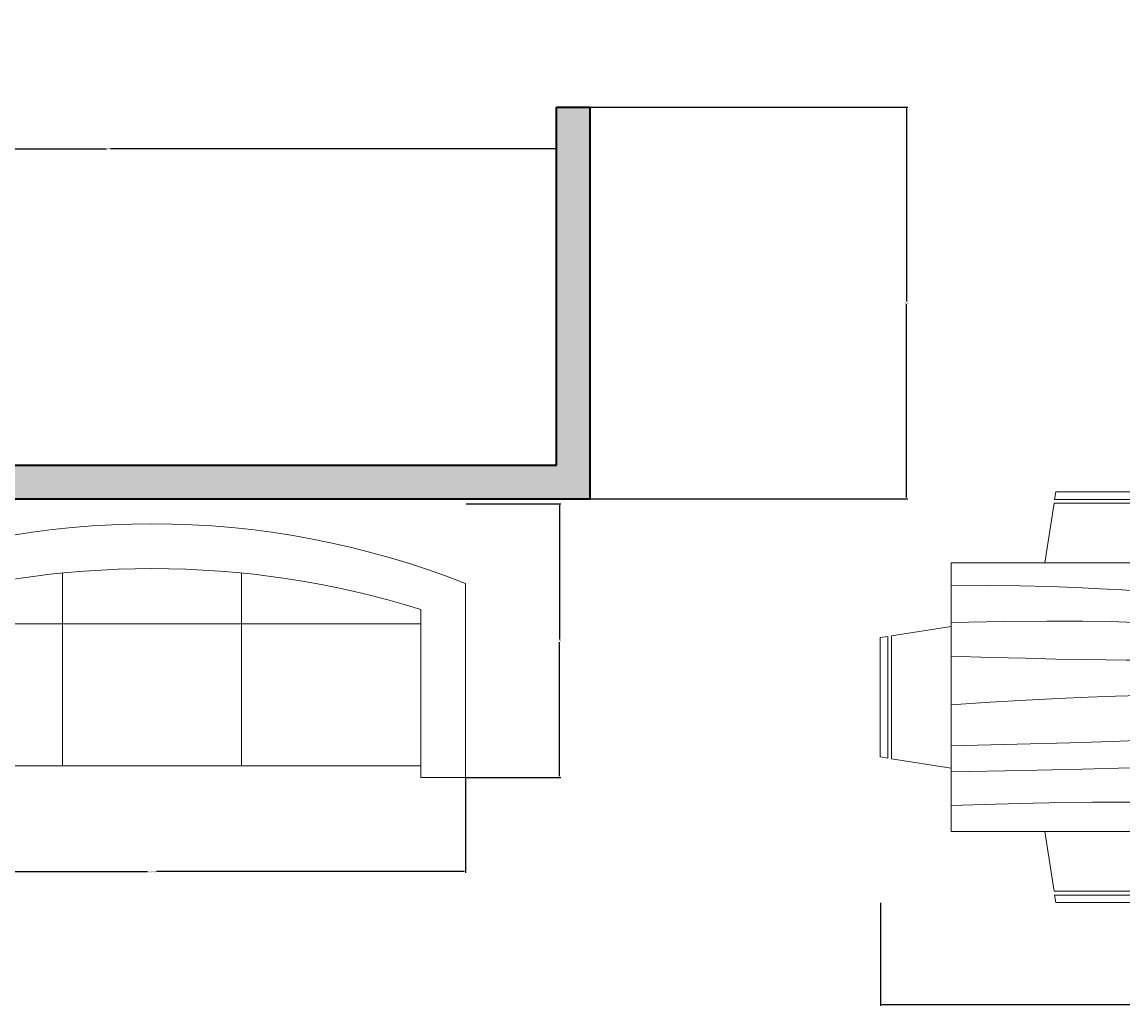
# Model space of a CAD drawing. Units: inches. Extents: x 1563 to 2428, y 777 to 1464.
# Tile 5 of 11: x 1663 to 1810, y 1130 to 1263. Entities that reach past the tile are written whole.
import ezdxf

# ---------------------------------------------------------------- set-up
doc = ezdxf.new("R2010")
doc.units = ezdxf.units.IN
for name, color, linetype, lineweight in [('A-ANNO-DIMS', 2, 'Continuous', 18), ('A-FURN', 9, 'Continuous', 18), ('A-WALL', 7, 'Continuous', 35), ('A-WALL-PATT', 8, 'Continuous', 13)]:
    doc.layers.add(name, color=color, linetype=linetype, lineweight=lineweight)
doc.styles.get("Standard").update_dxf_attribs({"font": 'arial.ttf'})
doc.dimstyles.get("Standard").update_dxf_attribs({"dimtxt": 0.18, "dimasz": 0.18, "dimexe": 0.18, "dimexo": 0.0625, "dimgap": 0.09, "dimtad": 0, "dimtih": 1, "dimtoh": 1, "dimdec": 4, "dimzin": 0, "dimdsep": 46, "dimtxsty": 'Standard', "dimcen": 0.09, "dimadec": 0, "dimazin": 0, "dimtfac": 1, "dimtdec": 4, "dimtofl": 0, "dimtmove": 0, "dimatfit": 3, "dimfxl": 1, "dimtolj": 1, "dimtzin": 0, "dimarcsym": 0})

# ---------------------------------------------------------------- blocks, each defined once
blk = doc.blocks.new('Sofa - Roundback 7 ft.')
for p, q in [((-12.00002, -32.4421), (-12.00003, -6.5971)), ((11.99997, -32.4421), (11.99998, -6.5971)), ((-36.000027, -34), (-36.000027, -11.4696)), ((35.99998, -34), (35.99998, -11.4696)), ((-35.999844, -13.3819), (35.9998, -13.3819)), ((-36.000027, -32.4421), (35.99998, -32.4421))]:
    blk.add_line(p, q)
for points in [[(-36.000027, -34), (-42.000027, -34), (-42.000027, -8)], [(41.99998, -8), (41.99998, -34), (35.99998, -34)]]:
    blk.add_lwpolyline(points)
for centre, radius, start, end in [((0, -114.25), 114.25, 68.43141, 111.5686), ((-0.00001, -127.1968), 121.1968, 72.72033, 107.2797)]:
    blk.add_arc(centre, radius, start, end)
blk = doc.blocks.new('Dining Set - 36 x 72 in.')
for p, q in [((-22, 27.5), (-22.1562, 26.50042)), ((-22, 27.5), (-6, 27.5)), ((-5.8437, 26.49966), (-6, 27.5)), ((6, 27.5), (5.8438, 26.50042)), ((6, 27.5), (22, 27.5)), ((22.1563, 26.49966), (22, 27.5)), ((-22.2343, 26.00059), (-23.4847, 17.99762)), ((-22.2304, 26), (-5.7608, 26)), ((-5.8416, 26.5), (-22.1534, 26.5)), ((-4.5152, 17.99762), (-5.7655, 25.99926)), ((5.7657, 26.00059), (4.5153, 17.99762)), ((5.7696, 26), (22.2392, 26)), ((22.1584, 26.5), (5.8466, 26.5)), ((23.4848, 17.99762), (22.2345, 25.99926)), ((36, 18), (-36, 18)), ((-36, 18), (-36, -18)), ((36, -18), (36, 18)), ((-44.0006, 8.23428), (-35.9976, 9.48474)), ((44.0006, 8.23428), (35.9976, 9.48474)), ((-45.5, 8), (-44.5004, 8.15617)), ((-45.5, 8), (-45.5, -8)), ((-44.5, -8.15843), (-44.5, 8.15338)), ((-44, 8.23041), (-44, -8.23915)), ((44, 8.23041), (44, -8.23915)), ((44.5, -8.15843), (44.5, 8.15338)), ((45.5, 8), (44.5005, 8.15617)), ((45.5, 8), (45.5, -8)), ((-44.4997, -8.15631), (-45.5, -8)), ((-35.9976, -9.48476), (-43.9993, -8.2345)), ((35.9976, -9.48476), (43.9993, -8.2345)), ((44.4997, -8.15631), (45.5, -8)), ((-36, -18), (36, -18)), ((-22.2343, -26.0006), (-23.4847, -17.99762)), ((-4.5152, -17.99762), (-5.7655, -25.99928)), ((5.7657, -26.0006), (4.5153, -17.99762)), ((23.4848, -17.99762), (22.2345, -25.99928)), ((-22.2304, -26), (-5.7608, -26)), ((-22, -27.5), (-22.1562, -26.50044)), ((-5.8416, -26.5), (-22.1534, -26.5)), ((-5.8437, -26.49967), (-6, -27.5)), ((5.7696, -26), (22.2392, -26)), ((6, -27.5), (5.8438, -26.50044)), ((22.1584, -26.5), (5.8466, -26.5)), ((22.1563, -26.49967), (22, -27.5)), ((-22, -27.5), (-6, -27.5)), ((6, -27.5), (22, -27.5))]:
    blk.add_line(p, q)
for points in [[(-36, 15), (-31.1772, 14.97754), (-26.8079, 14.91406), (-22.8538, 14.81543), (-19.276, 14.6875), (-16.0362, 14.53613), (-13.0957, 14.36718), (-10.4159, 14.18652), (-7.9583, 14), (-5.6904, 13.81315), (-3.6035, 13.63021), (-1.6954, 13.45508), (0.0365, 13.29166), (1.5945, 13.14388), (2.9811, 13.01562), (4.1988, 12.9108), (5.25, 12.83333), (6.1393, 12.78613), (6.8802, 12.76823), (7.4883, 12.77767), (7.9792, 12.8125), (8.3685, 12.87077), (8.6719, 12.95052), (8.9049, 13.0498), (9.0833, 13.16666), (9.2205, 13.29899), (9.3216, 13.44401), (9.3895, 13.59879), (9.4271, 13.76041), (9.4373, 13.92594), (9.4232, 14.09245), (9.3875, 14.257), (9.3333, 14.41666), (9.2638, 14.56917), (9.1836, 14.71484), (9.0975, 14.85465), (9.0104, 14.98958), (8.9272, 15.1206), (8.8529, 15.2487), (8.7922, 15.37483), (8.75, 15.5), (8.7305, 15.62467), (8.7344, 15.74739), (8.7617, 15.86621), (8.8125, 15.97916), (8.8867, 16.08431), (8.9844, 16.17968), (9.1055, 16.26334), (9.25, 16.33333), (9.4189, 16.38802), (9.6172, 16.42708), (9.8506, 16.45052), (10.125, 16.45833), (10.4463, 16.45052), (10.8203, 16.42708), (11.2529, 16.38802), (11.75, 16.33333), (12.3184, 16.26318), (12.9694, 16.17838), (13.7151, 16.07991), (14.5677, 15.96875), (15.5395, 15.84586), (16.6426, 15.71224), (17.8893, 15.56884), (19.2917, 15.41666), (20.859, 15.25667), (22.5879, 15.08984), (24.4721, 14.91715), (26.5052, 14.73958), (28.6809, 14.5581), (30.9929, 14.3737), (33.4347, 14.18733), (36, 14)], [(-36, 10), (-28.9766, 10.14274), (-23.1725, 10.20442), (-18.4241, 10.19775), (-14.5677, 10.13541), (-11.4399, 10.03011), (-8.877, 9.89453), (-6.7154, 9.74137), (-4.7917, 9.58333), (-2.9698, 9.43082), (-1.2246, 9.28515), (0.4415, 9.14534), (2.026, 9.01041), (3.5266, 8.87939), (4.9408, 8.7513), (6.266, 8.62516), (7.5, 8.5), (8.6411, 8.37549), (9.6914, 8.2539), (10.6538, 8.13818), (11.5312, 8.03125), (12.3267, 7.93603), (13.043, 7.85547), (13.6831, 7.79248), (14.25, 7.75), (14.7471, 7.7303), (15.1797, 7.73307), (15.5537, 7.75732), (15.875, 7.80208), (16.1494, 7.86637), (16.3828, 7.94922), (16.5811, 8.04964), (16.75, 8.16666), (16.8944, 8.29915), (17.0143, 8.44531), (17.1089, 8.60319), (17.1771, 8.77083), (17.218, 8.94629), (17.2305, 9.1276), (17.2137, 9.31282), (17.1667, 9.5), (17.0895, 9.6875), (16.987, 9.875), (16.8649, 10.0625), (16.7292, 10.25), (16.5856, 10.4375), (16.4401, 10.625), (16.2985, 10.8125), (16.1667, 11), (16.05, 11.18733), (15.9518, 11.3737), (15.8752, 11.5581), (15.8229, 11.73958), (15.798, 11.91715), (15.8034, 12.08984), (15.842, 12.25667), (15.9167, 12.41666), (16.0295, 12.56836), (16.1784, 12.70833), (16.3605, 12.83268), (16.5729, 12.9375), (16.8127, 13.01888), (17.0768, 13.07291), (17.3625, 13.0957), (17.6667, 13.08333), (17.9894, 13.03312), (18.3418, 12.94726), (18.7382, 12.82918), (19.1927, 12.68229), (19.7195, 12.51001), (20.3327, 12.31575), (21.0465, 12.10294), (21.875, 11.875), (22.8357, 11.63354), (23.959, 11.37304), (25.2786, 11.08618), (26.8282, 10.76562), (28.6414, 10.40405), (30.752, 9.99414), (33.1936, 9.52856), (36, 9)], [(-36, 5.5), (-30.7157, 5.3348), (-26.069, 5.20963), (-21.9946, 5.11767), (-18.4271, 5.05208), (-15.3009, 5.00602), (-12.5508, 4.97265), (-10.1112, 4.94515), (-7.9167, 4.91666), (-5.909, 4.88167), (-4.0586, 4.83984), (-2.3429, 4.79215), (-0.7396, 4.73958), (0.7739, 4.6831), (2.22, 4.6237), (3.6213, 4.56233), (5, 4.5), (6.373, 4.43782), (7.7344, 4.3776), (9.0723, 4.32129), (10.375, 4.27083), (11.6309, 4.22819), (12.8281, 4.19531), (13.9551, 4.17415), (15, 4.16666), (15.954, 4.17448), (16.819, 4.19791), (17.6001, 4.23698), (18.3021, 4.29166), (18.9299, 4.36198), (19.4883, 4.44791), (19.9823, 4.54948), (20.4167, 4.66666), (20.7969, 4.79899), (21.1302, 4.94401), (21.4245, 5.09879), (21.6875, 5.26041), (21.9271, 5.42594), (22.1511, 5.59245), (22.3672, 5.757), (22.5834, 5.91666), (22.8065, 6.06868), (23.0404, 6.21093), (23.2879, 6.34147), (23.5521, 6.45833), (23.8358, 6.55957), (24.142, 6.64323), (24.4735, 6.70735), (24.8334, 6.75), (25.2235, 6.76969), (25.642, 6.76692), (26.0858, 6.74267), (26.5521, 6.69791), (27.0379, 6.63362), (27.5404, 6.55078), (28.0565, 6.45036), (28.5834, 6.33333), (29.1242, 6.19987), (29.7071, 6.04687), (30.3661, 5.87044), (31.1354, 5.66666), (32.0493, 5.43164), (33.142, 5.16146), (34.4475, 4.85221), (36, 4.5)], [(-36, -1), (-30.7915, -0.6591), (-26.0195, -0.38216), (-21.6519, -0.16284), (-17.6563, 0.00521), (-14.0005, 0.12833), (-10.6523, 0.21289), (-7.5796, 0.26522), (-4.75, 0.29166), (-2.134, 0.29793), (0.2878, 0.28711), (2.5317, 0.26163), (4.6146, 0.22396), (6.5529, 0.17651), (8.3633, 0.12174), (10.0623, 0.06209), (11.6667, 0), (13.1899, -0.06201), (14.6341, -0.1211), (15.9982, -0.17432), (17.2813, -0.21875), (18.4823, -0.25147), (19.6003, -0.26953), (20.6343, -0.27002), (21.5834, -0.25), (22.4481, -0.20768), (23.2357, -0.14584), (23.9549, -0.06836), (24.6146, 0.02083), (25.2235, 0.11784), (25.7904, 0.21875), (26.3241, 0.31966), (26.8334, 0.41666), (27.3265, 0.50618), (27.8099, 0.58593), (28.2894, 0.65397), (28.7709, 0.70833), (29.2601, 0.74707), (29.763, 0.76823), (30.2855, 0.76985), (30.8334, 0.75), (31.4088, 0.70784), (31.9994, 0.64713), (32.589, 0.57275), (33.1615, 0.48958), (33.7008, 0.4025), (34.1908, 0.3164), (34.6153, 0.23616), (34.9584, 0.16666), (35.2099, 0.11165), (35.3848, 0.07031), (35.504, 0.04069), (35.5886, 0.02083), (35.6594, 0.00879), (35.7377, 0.0026), (35.8442, 0.00032), (36, 0)], [(-36, -6.5), (-27.1843, -6.31267), (-20.084, -6.1263), (-14.469, -5.9419), (-10.1094, -5.76042), (-6.7752, -5.58285), (-4.2363, -5.41016), (-2.2629, -5.24333), (-0.625, -5.08334), (0.8708, -4.93099), (2.2715, -4.78646), (3.5872, -4.64974), (4.8281, -4.52084), (6.0046, -4.39974), (7.127, -4.28646), (8.2053, -4.18099), (9.25, -4.08334), (10.2705, -3.99382), (11.2734, -3.91407), (12.2647, -3.84603), (13.25, -3.79167), (14.2354, -3.75293), (15.2266, -3.73177), (16.2295, -3.73015), (17.25, -3.75), (18.2912, -3.79248), (19.3451, -3.85547), (20.4009, -3.93604), (21.4479, -4.03125), (22.4754, -4.13819), (23.4727, -4.25391), (24.4289, -4.37549), (25.3334, -4.5), (26.1785, -4.62492), (26.9694, -4.74935), (27.7145, -4.87281), (28.4219, -4.99479), (29.1, -5.11483), (29.7572, -5.23242), (30.4016, -5.34709), (31.0417, -5.45834), (31.6837, -5.56437), (32.3262, -5.65821), (32.9658, -5.73153), (33.599, -5.77604), (34.2224, -5.78345), (34.8327, -5.74545), (35.4264, -5.65373), (36, -5.5)], [(-36, -10), (-26.4022, -9.81299), (-18.4675, -9.62891), (-11.9839, -9.45069), (-6.7396, -9.28125), (-2.5226, -9.12354), (0.8789, -8.98047), (3.6769, -8.85498), (6.0833, -8.75), (8.2767, -8.66765), (10.3021, -8.60677), (12.1712, -8.56543), (13.8958, -8.54167), (15.4876, -8.53353), (16.9583, -8.53907), (18.3197, -8.55632), (19.5834, -8.58334), (20.7616, -8.61841), (21.8685, -8.66081), (22.9188, -8.71004), (23.9271, -8.76563), (24.9081, -8.82707), (25.8763, -8.89388), (26.8465, -8.96558), (27.8334, -9.04167), (28.8474, -9.12118), (29.8828, -9.20117), (30.93, -9.27824), (31.9792, -9.34896), (33.0205, -9.40991), (34.0443, -9.45768), (35.0407, -9.48885), (36, -9.5)], [(-36, -14.5), (-30.0881, -14.33513), (-25.0332, -14.21224), (-20.7312, -14.12647), (-17.0781, -14.07292), (-13.97, -14.04671), (-11.3027, -14.04297), (-8.9724, -14.05681), (-6.875, -14.08334), (-4.9224, -14.11833), (-3.0905, -14.16016), (-1.3709, -14.20785), (0.2448, -14.26042), (1.7647, -14.3169), (3.1973, -14.3763), (4.5507, -14.43767), (5.8333, -14.5), (7.0554, -14.5621), (8.235, -14.62175), (9.3922, -14.67652), (10.5469, -14.72396), (11.7192, -14.76164), (12.929, -14.78711), (14.1965, -14.79794), (15.5417, -14.79167), (16.9933, -14.76424), (18.6152, -14.70508), (20.4804, -14.60197), (22.6615, -14.44271), (25.2312, -14.21509), (28.2624, -13.9069), (31.8277, -13.50594), (36, -13)]]:
    blk.add_lwpolyline(points)
blk = doc.blocks.new('*D24')
at = {"layer": 'A-ANNO-DIMS', "color": 0, "lineweight": -2, "transparency": 16777216}
for p, q in [((1637.93, 1162.02), (1637.93, 1149.31)), ((1721.93, 1162.02), (1721.93, 1149.31)), ((1638.11, 1149.49), (1679.34, 1149.49)), ((1721.75, 1149.49), (1680.53, 1149.49))]:
    blk.add_line(p, q, dxfattribs=at)
at = {"layer": 'A-ANNO-DIMS', "color": 0, "transparency": 16777216}
for points in [[(1638.11, 1149.52), (1638.11, 1149.46), (1637.93, 1149.49)], [(1721.75, 1149.52), (1721.75, 1149.46), (1721.93, 1149.49)]]:
    blk.add_solid(points, dxfattribs=at)
at = {"layer": 'Defpoints', "color": 0, "transparency": 16777216}
for p in [(1637.93, 1162.09), (1721.93, 1162.09), (1721.93, 1149.49)]:
    blk.add_point(p, dxfattribs=at)
at = {"layer": 'A-ANNO-DIMS', "color": 0, "transparency": 16777216, "insert": (1679.93, 1149.49), "char_height": 0.18, "attachment_point": 5}
blk.add_mtext('\\A1;SOFA 84', dxfattribs=at)
blk = doc.blocks.new('*D25')
at = {"layer": 'A-ANNO-DIMS', "color": 0, "lineweight": -2, "transparency": 16777216}
for p, q in [((1721.99, 1198.75), (1734.71, 1198.75)), ((1734.53, 1198.57), (1734.53, 1180.6)), ((1734.53, 1162.27), (1734.53, 1180.24)), ((1721.99, 1162.09), (1734.71, 1162.09))]:
    blk.add_line(p, q, dxfattribs=at)
at = {"layer": 'A-ANNO-DIMS', "color": 0, "transparency": 16777216}
for points in [[(1734.5, 1198.57), (1734.56, 1198.57), (1734.53, 1198.75)], [(1734.5, 1162.27), (1734.56, 1162.27), (1734.53, 1162.09)]]:
    blk.add_solid(points, dxfattribs=at)
at = {"layer": 'Defpoints', "color": 0, "transparency": 16777216}
for p in [(1721.93, 1198.75), (1734.53, 1198.75), (1721.93, 1162.09)]:
    blk.add_point(p, dxfattribs=at)
at = {"layer": 'A-ANNO-DIMS', "color": 0, "transparency": 16777216, "insert": (1734.53, 1180.42), "char_height": 0.18, "attachment_point": 5}
blk.add_mtext('\\A1;37', dxfattribs=at)
blk = doc.blocks.new('*D42')
at = {"layer": 'A-ANNO-DIMS', "color": 0, "lineweight": -2, "transparency": 16777216}
for p, q in [((1777.49, 1145.29), (1777.49, 1131.52)), ((1868.49, 1145.29), (1868.49, 1131.52)), ((1777.67, 1131.7), (1822.03, 1131.7)), ((1868.31, 1131.7), (1823.94, 1131.7))]:
    blk.add_line(p, q, dxfattribs=at)
at = {"layer": 'A-ANNO-DIMS', "color": 0, "transparency": 16777216}
for points in [[(1777.67, 1131.73), (1777.67, 1131.67), (1777.49, 1131.7)], [(1868.31, 1131.73), (1868.31, 1131.67), (1868.49, 1131.7)]]:
    blk.add_solid(points, dxfattribs=at)
at = {"layer": 'Defpoints', "color": 0, "transparency": 16777216}
for p in [(1777.49, 1145.35), (1868.49, 1145.35), (1868.49, 1131.7)]:
    blk.add_point(p, dxfattribs=at)
at = {"layer": 'A-ANNO-DIMS', "color": 0, "transparency": 16777216, "insert": (1822.99, 1131.7), "char_height": 0.18, "attachment_point": 5}
blk.add_mtext('\\A1;DINING SET 91', dxfattribs=at)
blk = doc.blocks.new('*D56')
at = {"layer": 'A-ANNO-DIMS', "color": 0, "lineweight": -2, "transparency": 16777216}
for p, q in [((1614.11, 1203.99), (1614.11, 1246.51)), ((1734.11, 1203.99), (1734.11, 1246.51)), ((1614.29, 1246.33), (1673.83, 1246.33)), ((1733.93, 1246.33), (1674.39, 1246.33))]:
    blk.add_line(p, q, dxfattribs=at)
at = {"layer": 'A-ANNO-DIMS', "color": 0, "transparency": 16777216}
for points in [[(1614.29, 1246.36), (1614.29, 1246.3), (1614.11, 1246.33)], [(1733.93, 1246.36), (1733.93, 1246.3), (1734.11, 1246.33)]]:
    blk.add_solid(points, dxfattribs=at)
at = {"layer": 'Defpoints', "color": 0, "transparency": 16777216}
for p in [(1734.11, 1246.33), (1614.11, 1203.93), (1734.11, 1203.93)]:
    blk.add_point(p, dxfattribs=at)
at = {"layer": 'A-ANNO-DIMS', "color": 0, "transparency": 16777216, "insert": (1674.11, 1246.33), "char_height": 0.18, "attachment_point": 5}
blk.add_mtext('\\A1;120', dxfattribs=at)
blk = doc.blocks.new('*D57')
at = {"layer": 'A-ANNO-DIMS', "color": 0, "lineweight": -2, "transparency": 16777216}
for p, q in [((1738.67, 1251.93), (1781.19, 1251.93)), ((1781.01, 1251.75), (1781.01, 1225.86)), ((1781.01, 1199.61), (1781.01, 1225.5)), ((1738.67, 1199.43), (1781.19, 1199.43))]:
    blk.add_line(p, q, dxfattribs=at)
at = {"layer": 'A-ANNO-DIMS', "color": 0, "transparency": 16777216}
for points in [[(1780.98, 1251.75), (1781.04, 1251.75), (1781.01, 1251.93)], [(1780.98, 1199.61), (1781.04, 1199.61), (1781.01, 1199.43)]]:
    blk.add_solid(points, dxfattribs=at)
at = {"layer": 'Defpoints', "color": 0, "transparency": 16777216}
for p in [(1738.61, 1251.93), (1738.61, 1199.43), (1781.01, 1199.43)]:
    blk.add_point(p, dxfattribs=at)
at = {"layer": 'A-ANNO-DIMS', "color": 0, "transparency": 16777216, "insert": (1781.01, 1225.68), "char_height": 0.18, "attachment_point": 5}
blk.add_mtext('\\A1;52.5', dxfattribs=at)

msp = doc.modelspace()

# ---------------------------------------------------------------- hatches: boundary and pattern name
at = {"layer": 'A-WALL-PATT'}
h = msp.add_hatch(color=256, dxfattribs=at)
h.dxf.hatch_style = 1
h.paths.add_polyline_path([(1965.105, 1421.428), (1605.105, 1421.428), (1605.105, 821.428), (1965.105, 821.428)])
h.paths.add_polyline_path([(1614.105, 1199.428), (1704.105, 1199.428), (1738.605, 1199.428), (1738.605, 1251.928), (1734.105, 1251.928), (1734.105, 1203.928), (1704.105, 1203.928), (1614.105, 1203.928), (1614.105, 1335.928), (1665.105, 1335.928), (1665.105, 1340.428), (1614.105, 1340.428), (1614.105, 1412.428), (1704.105, 1412.428), (1704.105, 1340.428), (1701.105, 1340.428), (1701.105, 1335.928), (1704.105, 1335.928), (1768.605, 1335.928), (1768.605, 1340.428), (1708.605, 1340.428), (1708.605, 1412.428), (1807.605, 1412.428), (1807.605, 1340.428), (1804.605, 1340.428), (1804.605, 1335.928), (1807.605, 1335.928), (1807.605, 1275.928), (1815.105, 1275.928), (1815.105, 1280.428), (1812.105, 1280.428), (1812.105, 1412.428), (1956.105, 1412.428), (1956.105, 1280.428), (1854.105, 1280.428), (1854.105, 1275.928), (1956.105, 1275.928), (1956.105, 830.428), (1614.105, 830.428)], flags=16)
h.paths.add_polyline_path([(1917.224, 1038.928), (1917.224, 1043.846, -0.4014527), (1951.591, 1079.751), (1951.591, 1079.786), (1953.163, 1079.786), (1953.163, 1043.846), (1953.163, 1038.455), (1953.105, 1034.428), (1953.105, 1038.928), (1953.163, 1043.846), (1951.591, 1043.846), (1951.591, 1079.751, 0.4014527), (1917.224, 1043.846), (1917.224, 1038.455), (1917.224, 1034.428), (1834.605, 1034.428), (1834.605, 906.928), (1858.605, 906.928), (1858.605, 954.928), (1932.105, 954.928), (1932.105, 902.428), (1834.605, 902.428), (1834.605, 1034.428), (1914.224, 1034.428), (1914.224, 1038.928)], flags=0)
edge = h.paths.add_edge_path(flags=0)
edge.add_ellipse((1674.345, 1004.483), major_axis=(1.48, 0), ratio=0.8423039, start_angle=90, end_angle=180, ccw=False)
edge.add_line((1674.345, 1005.73), (1674.921, 1005.73))
edge.add_ellipse((2202.617, 985.642), major_axis=(528.234, 0), ratio=0.8423039, start_angle=176.34957, end_angle=177.82005, ccw=False)
edge.add_ellipse((1739.278, 760.804), major_axis=(-313.308, 0), ratio=0.8423039, start_angle=-77.87403, end_angle=-76.21947, ccw=False)
edge.add_ellipse((1739.278, 767.659), major_axis=(305.303, 0), ratio=0.8423039, start_angle=100.20954, end_angle=102.44463, ccw=False)
edge.add_ellipse((1659.357, 1231.328), major_axis=(250.96, 0), ratio=0.8423039, start_angle=-80.74343, end_angle=-77.44507)
edge.add_line((1705.625, 1023.567), (1711.685, 1026.918))
edge.add_ellipse((1711.754, 1026.21), major_axis=(0.74, 0), ratio=0.8423039, start_angle=52.06687, end_angle=90, ccw=False)
edge.add_line((1712.16, 1026.731), (1717.882, 1023.567))
edge.add_ellipse((1764.151, 1231.328), major_axis=(250.96, 0), ratio=0.8423039, start_angle=257.44507, end_angle=260.74343)
edge.add_ellipse((1684.229, 767.659), major_axis=(305.303, 0), ratio=0.8423039, start_angle=77.55537, end_angle=79.79046, ccw=False)
edge.add_ellipse((1684.229, 760.804), major_axis=(-313.308, 0), ratio=0.8423039, start_angle=256.21947, end_angle=257.87403, ccw=False)
edge.add_ellipse((1220.891, 985.642), major_axis=(-528.234, 0), ratio=0.8423039, start_angle=182.17995, end_angle=183.65043, ccw=False)
edge.add_line((1748.586, 1005.73), (1749.162, 1005.73))
edge.add_ellipse((1749.162, 1004.483), major_axis=(-1.48, 0), ratio=0.8423039, start_angle=180, end_angle=270, ccw=False)
edge.add_line((1750.642, 1004.483), (1750.642, 980.28))
edge.add_ellipse((1749.162, 980.28), major_axis=(1.48, 0), ratio=0.8423039, start_angle=270, end_angle=360, ccw=False)
edge.add_ellipse((-8843.864, 962.352), major_axis=(10593.026, 0), ratio=0.84230387, start_angle=-0.3241203, end_angle=0.0902291, ccw=False)
edge.add_ellipse((-8843.864, 962.352), major_axis=(10593.026, 0), ratio=0.84230387, start_angle=-0.3838668, end_angle=-0.3241203, ccw=False)
edge.add_ellipse((1749.162, 890.136), major_axis=(1.48, 0), ratio=0.8423039, start_angle=0, end_angle=90, ccw=False)
edge.add_line((1750.642, 890.136), (1750.642, 865.933))
edge.add_ellipse((1749.162, 865.933), major_axis=(1.48, 0), ratio=0.8423039, start_angle=270, end_angle=360, ccw=False)
edge.add_line((1749.162, 864.686), (1748.528, 864.686))
edge.add_ellipse((-8843.864, 962.352), major_axis=(10593.026, 0), ratio=0.84230387, start_angle=-0.6186432, end_angle=-0.5282715, ccw=False)
edge.add_ellipse((1747.592, 846.206), major_axis=(-2.22, 0), ratio=0.8423039, start_angle=179.37176, end_angle=248.46476, ccw=False)
edge.add_ellipse((-8844.604, 962.352), major_axis=(-10595.313, 0), ratio=0.842303864, start_angle=179.3534459, end_angle=179.3717628, ccw=False)
edge.add_ellipse((1744.512, 842.854), major_axis=(-5.246, 0), ratio=0.8423039, start_angle=90, end_angle=179.35345, ccw=False)
edge.add_line((1744.512, 838.435), (1678.995, 838.435))
edge.add_ellipse((1678.995, 842.854), major_axis=(5.246, 0), ratio=0.8423039, start_angle=180.64655, end_angle=270, ccw=False)
edge.add_ellipse((12268.111, 962.352), major_axis=(-10595.313, 0), ratio=0.84230387, start_angle=0.6282372, end_angle=0.6465541, ccw=False)
edge.add_ellipse((1675.916, 846.206), major_axis=(-2.22, 0), ratio=0.8423039, start_angle=-68.46476, end_angle=0.62824, ccw=False)
edge.add_ellipse((12267.371, 962.352), major_axis=(-10593.026, 0), ratio=0.84230387, start_angle=0.5282715, end_angle=0.6465541, ccw=False)
edge.add_line((1674.98, 864.686), (1674.345, 864.686))
edge.add_ellipse((1674.345, 865.933), major_axis=(-1.48, 0), ratio=0.8423039, start_angle=0, end_angle=90, ccw=False)
edge.add_line((1672.865, 865.933), (1672.865, 890.136))
edge.add_ellipse((1674.345, 890.136), major_axis=(1.48, 0), ratio=0.8423039, start_angle=90, end_angle=180, ccw=False)
edge.add_ellipse((12267.371, 962.352), major_axis=(-10593.026, 0), ratio=0.84230387, start_angle=0.3241203, end_angle=0.3838668, ccw=False)
edge.add_ellipse((12267.371, 962.352), major_axis=(-10593.026, 0), ratio=0.84230387, start_angle=-0.0902291, end_angle=0.3241203, ccw=False)
edge.add_ellipse((1674.345, 980.28), major_axis=(-1.48, 0), ratio=0.8423039, start_angle=0, end_angle=90, ccw=False)
edge.add_line((1672.865, 980.28), (1672.865, 1004.483))
h.paths.add_polyline_path([(1622.542, 1135.584), (1648.534, 1136.233), (1648.683, 1130.234), (1647.126, 1130.196), (1648.323, 1082.21), (1649.88, 1082.249), (1650.03, 1076.251), (1624.038, 1075.603, -0.266667)], flags=0)
edge = h.paths.add_edge_path(flags=0)
edge.add_line((1694.584, 990.705), (1700.334, 994.711))
edge.add_line((1700.334, 994.711), (1702.248, 994.711))
edge.add_line((1702.248, 994.711), (1702.248, 997.061))
edge.add_ellipse((1758.417, 997.061), major_axis=(56.169, 0), ratio=0.8423039, start_angle=150.56143, end_angle=180, ccw=False)
edge.add_ellipse((1665.091, 997.061), major_axis=(-56.169, 0), ratio=0.8423039, start_angle=180, end_angle=209.43857, ccw=False)
edge.add_line((1721.26, 997.061), (1721.26, 994.711))
edge.add_line((1721.26, 994.711), (1723.174, 994.711))
edge.add_line((1723.174, 994.711), (1728.923, 990.705))
edge.add_line((1728.923, 990.705), (1728.923, 975.895))
edge.add_ellipse((1725.091, 976.043), major_axis=(0.357, 6.34), ratio=0.6038336, start_angle=106.34259, end_angle=270.99799, ccw=False)
edge.add_line((1721.26, 975.15), (1721.26, 997.061))
edge.add_ellipse((1665.091, 997.061), major_axis=(-56.169, 0), ratio=0.8423039, start_angle=180, end_angle=209.43857)
edge.add_ellipse((1758.417, 997.061), major_axis=(56.169, 0), ratio=0.8423039, start_angle=150.56143, end_angle=180)
edge.add_line((1702.248, 997.061), (1702.248, 975.15))
edge.add_ellipse((1698.416, 976.043), major_axis=(-0.357, 6.34), ratio=0.6038336, start_angle=89.00201, end_angle=253.65741, ccw=False)
edge.add_line((1694.584, 975.895), (1694.584, 990.705))
edge = h.paths.add_edge_path(flags=0)
edge.add_line((1675.832, 952.075), (1679.883, 938.848))
edge.add_ellipse((5378.107, 931.045), major_axis=(-3698.236, 0), ratio=0.84230387, start_angle=-0.120897, end_angle=0.364076)
edge.add_line((1679.976, 907.545), (1676.149, 892.52))
edge.add_ellipse((12267.371, 962.352), major_axis=(10591.546, 0), ratio=0.84230387, start_angle=180.3241656, end_angle=180.3777642, ccw=False)
edge.add_ellipse((12267.371, 962.352), major_axis=(10591.546, 0), ratio=0.84230387, start_angle=180.0555943, end_angle=180.3241656, ccw=False)
edge = h.paths.add_edge_path(flags=0)
edge.add_ellipse((1706.366, 891.542), major_axis=(81.773, 0), ratio=0.8423039, start_angle=94.27742, end_angle=111.83495, ccw=False)
edge.add_line((1701.225, 960.283), (1722.283, 960.283))
edge.add_ellipse((1717.141, 891.542), major_axis=(-81.773, 0), ratio=0.8423039, start_angle=248.16505, end_angle=265.72258, ccw=False)
edge.add_line((1743.29, 956.803), (1741.105, 940.427))
edge.add_ellipse((1714.553, 877.238), major_axis=(79.58, 0), ratio=0.8423039, start_angle=67.20809, end_angle=85.12993)
edge.add_line((1720.25, 944.097), (1703.258, 944.097))
edge.add_ellipse((1708.954, 877.238), major_axis=(79.58, 0), ratio=0.8423039, start_angle=94.87007, end_angle=112.79191)
edge.add_line((1682.403, 940.427), (1680.218, 956.803))
h.paths.add_polyline_path([(1664.992, 1093.991), (1664.992, 1123.991), (1724.992, 1123.991), (1724.992, 1093.991)], flags=0)
h.paths.add_polyline_path([(1716.588, 1099.729), (1715.404, 1099.805), (1715.021, 1099.823), (1716.177, 1099.758)], flags=0)
h.paths.add_polyline_path([(1711.325, 1103.757), (1712.167, 1103.706), (1713.009, 1103.642), (1713.84, 1103.566), (1715.041, 1103.439), (1716.532, 1103.244), (1717.793, 1103.048), (1718.876, 1102.854), (1719.676, 1102.699), (1720.157, 1102.605), (1720.632, 1102.513), (1721.109, 1102.424), (1721.595, 1102.339), (1722.088, 1102.264), (1722.585, 1102.205), (1723.082, 1102.17), (1723.575, 1102.164), (1724.321, 1102.211), (1724.533, 1102.268), (1723.842, 1102.16), (1722.864, 1102.172), (1721.894, 1102.287), (1720.935, 1102.454), (1720.157, 1102.605), (1719.676, 1102.699), (1719.18, 1102.795), (1718.66, 1102.892), (1718.109, 1102.991), (1717.517, 1103.091), (1716.876, 1103.191), (1716.179, 1103.29), (1715.435, 1103.387), (1714.652, 1103.48), (1713.84, 1103.566), (1713.009, 1103.642), (1712.167, 1103.706), (1711.325, 1103.757), (1710.492, 1103.791), (1709.676, 1103.806), (1708.873, 1103.805), (1707.707, 1103.78), (1707.292, 1103.757), (1708.499, 1103.805), (1710.086, 1103.807)], flags=0)
h.paths.add_polyline_path([(1713.959, 1106.591), (1714.651, 1106.624), (1715.279, 1106.674), (1715.852, 1106.736), (1716.373, 1106.807), (1716.851, 1106.885), (1717.289, 1106.966), (1717.696, 1107.046), (1718.341, 1107.178), (1719.173, 1107.331), (1720.169, 1107.421), (1721.131, 1107.383), (1722.032, 1107.286), (1722.934, 1107.152), (1723.887, 1106.983), (1724.746, 1106.795), (1724.72, 1106.798), (1724.663, 1106.807), (1724.241, 1106.906), (1724.159, 1106.924), (1723.885, 1106.979), (1723.546, 1107.044), (1723.157, 1107.113), (1722.732, 1107.182), (1722.284, 1107.249), (1721.827, 1107.308), (1721.375, 1107.357), (1720.942, 1107.391), (1720.539, 1107.406), (1720.162, 1107.405), (1719.804, 1107.388), (1719.459, 1107.357), (1719.12, 1107.314), (1718.781, 1107.259), (1718.435, 1107.195), (1718.076, 1107.124), (1717.402, 1106.986), (1716.59, 1106.837), (1715.56, 1106.696), (1714.317, 1106.598)], flags=0)
h.paths.add_polyline_path([(1708.692, 1110.124), (1709.455, 1110.13), (1710.147, 1110.149), (1710.772, 1110.18), (1711.334, 1110.224), (1711.836, 1110.28), (1712.283, 1110.349), (1712.678, 1110.43), (1713.026, 1110.524), (1713.33, 1110.63), (1713.596, 1110.746), (1713.832, 1110.87), (1714.042, 1110.999), (1714.234, 1111.131), (1714.413, 1111.264), (1714.586, 1111.396), (1715.065, 1111.75), (1715.879, 1112.11), (1716.842, 1112.224), (1717.903, 1112.165), (1719.048, 1111.965), (1719.867, 1111.736), (1720.686, 1111.487), (1721.596, 1111.22), (1721.917, 1111.136), (1721.028, 1111.383), (1720.222, 1111.628), (1719.815, 1111.75), (1719.434, 1111.857), (1719.054, 1111.951), (1718.672, 1112.031), (1718.292, 1112.097), (1717.918, 1112.149), (1717.554, 1112.185), (1717.204, 1112.204), (1716.871, 1112.206), (1716.559, 1112.191), (1716.271, 1112.156), (1716.006, 1112.105), (1715.761, 1112.038), (1715.534, 1111.957), (1715.323, 1111.864), (1715.125, 1111.759), (1714.937, 1111.645), (1714.759, 1111.524), (1714.586, 1111.396), (1714.413, 1111.264), (1714.003, 1110.96), (1713.331, 1110.606), (1712.501, 1110.382), (1711.61, 1110.245), (1710.489, 1110.158), (1709.111, 1110.121)], flags=0)
h.paths.add_polyline_path([(1707.127, 1113.075), (1707.639, 1113.025), (1708.092, 1112.991), (1708.49, 1112.975), (1708.836, 1112.977), (1709.135, 1112.996), (1709.392, 1113.032), (1709.612, 1113.084), (1709.798, 1113.15), (1709.957, 1113.23), (1710.092, 1113.324), (1710.208, 1113.431), (1710.304, 1113.554), (1710.379, 1113.698), (1710.434, 1113.866), (1710.467, 1114.062), (1710.477, 1114.289), (1710.463, 1114.553), (1710.426, 1114.857), (1710.364, 1115.202), (1710.282, 1115.58), (1710.184, 1115.98), (1710.076, 1116.391), (1709.961, 1116.801), (1709.844, 1117.201), (1709.731, 1117.579), (1709.626, 1117.924), (1709.532, 1118.228), (1709.454, 1118.493), (1709.392, 1118.723), (1709.351, 1118.924), (1709.293, 1119.435), (1709.831, 1119.942), (1710.705, 1120.121), (1711.507, 1119.898), (1712.224, 1119.567), (1713.189, 1119.016), (1713.529, 1118.804), (1712.958, 1119.148), (1712.468, 1119.428), (1712.046, 1119.649), (1711.683, 1119.817), (1711.366, 1119.937), (1711.084, 1120.016), (1710.826, 1120.057), (1710.582, 1120.067), (1710.354, 1120.049), (1710.142, 1120.006), (1709.951, 1119.941), (1709.781, 1119.857), (1709.635, 1119.757), (1709.516, 1119.645), (1709.426, 1119.524), (1709.366, 1119.395), (1709.335, 1119.255), (1709.331, 1119.1), (1709.351, 1118.924), (1709.392, 1118.723), (1709.454, 1118.493), (1709.52, 1118.268), (1709.799, 1117.356), (1710.028, 1116.57), (1710.245, 1115.749), (1710.45, 1114.804), (1710.477, 1114.289), (1710.448, 1113.654), (1709.908, 1113.153), (1709.165, 1112.979), (1708.318, 1112.974), (1707.448, 1113.039)], flags=0)
h.paths.add_polyline_path([(1700.892, 1119.857), (1701.604, 1119.819), (1702.196, 1119.805), (1702.683, 1119.813), (1703.076, 1119.841), (1703.387, 1119.887), (1703.63, 1119.951), (1703.816, 1120.03), (1703.959, 1120.124), (1704.069, 1120.23), (1704.15, 1120.346), (1704.204, 1120.47), (1704.234, 1120.599), (1704.242, 1120.731), (1704.231, 1120.864), (1704.202, 1120.996), (1704.159, 1121.124), (1704.103, 1121.246), (1704.039, 1121.362), (1703.97, 1121.474), (1703.901, 1121.582), (1703.834, 1121.687), (1703.775, 1121.79), (1703.564, 1122.226), (1704.048, 1122.698), (1704.756, 1122.769), (1705.49, 1122.723), (1706.24, 1122.641), (1706.547, 1122.601), (1706.092, 1122.657), (1705.695, 1122.701), (1705.348, 1122.732), (1705.049, 1122.751), (1704.792, 1122.757), (1704.573, 1122.751), (1704.386, 1122.732), (1704.227, 1122.701), (1704.092, 1122.657), (1703.977, 1122.601), (1703.88, 1122.534), (1703.802, 1122.458), (1703.742, 1122.374), (1703.702, 1122.284), (1703.68, 1122.188), (1703.677, 1122.09), (1703.692, 1121.991), (1703.726, 1121.89), (1703.769, 1121.802), (1704.039, 1121.362), (1704.301, 1120.887), (1704.133, 1120.165), (1703.43, 1119.866), (1702.481, 1119.798), (1701.306, 1119.827)], flags=0)
edge = h.paths.add_edge_path(flags=0)
edge.add_ellipse((1711.754, 1009.752), major_axis=(-147.018, 0), ratio=0.8423039, start_angle=76.40187, end_angle=103.59813)
edge.add_line((1741.105, 888.411), (1741.105, 869.587))
edge.add_ellipse((1711.754, 990.928), major_axis=(-147.018, 0), ratio=0.8423039, start_angle=76.40187, end_angle=103.59813, ccw=False)
edge.add_line((1682.403, 869.587), (1682.403, 888.411))
edge = h.paths.add_edge_path(flags=0)
edge.add_ellipse((-8843.864, 962.352), major_axis=(-10591.546, 0), ratio=0.84230387, start_angle=179.6758344, end_angle=179.9444057, ccw=False)
edge.add_ellipse((-8843.864, 962.352), major_axis=(-10591.546, 0), ratio=0.84230387, start_angle=179.6222358, end_angle=179.6758344, ccw=False)
edge.add_line((1747.358, 892.52), (1743.531, 907.545))
edge.add_ellipse((-1954.6, 931.045), major_axis=(3698.236, 0), ratio=0.84230387, start_angle=-0.364076, end_angle=0.120897)
edge.add_line((1743.625, 938.848), (1747.676, 952.075))
h.paths.add_polyline_path([(1637.931, 1162.087), (1637.931, 1188.087, -0.1904762), (1721.931, 1188.087), (1721.931, 1162.087), (1715.931, 1162.087), (1715.931, 1163.644), (1643.931, 1163.644), (1643.931, 1162.087)], flags=0)
h.paths.add_polyline_path([(1667.931, 1189.491, -0.0496282), (1691.931, 1189.491), (1691.931, 1182.705), (1667.931, 1182.705)], flags=0)
edge = h.paths.add_edge_path(flags=0)
edge.add_ellipse((1685.362, 859.825), major_axis=(-2.96, 0), ratio=0.8423039, start_angle=-90, end_angle=0, ccw=False)
edge.add_line((1685.362, 862.318), (1738.145, 862.318))
edge.add_ellipse((1738.145, 859.825), major_axis=(2.96, 0), ratio=0.8423039, start_angle=0, end_angle=90, ccw=False)
edge.add_line((1741.105, 859.825), (1741.105, 840.361))
edge.add_line((1741.105, 840.361), (1682.403, 840.361))
edge.add_line((1682.403, 840.361), (1682.403, 859.825))
h.paths.add_polyline_path([(1777.486, 1164.853), (1777.486, 1180.853), (1778.486, 1181.01), (1778.486, 1164.697)], flags=0)
h.paths.add_polyline_path([(1786.986, 1154.853), (1786.986, 1163.369), (1778.986, 1164.619), (1778.986, 1181.088), (1786.986, 1182.338), (1786.986, 1190.853), (1799.502, 1190.853), (1800.752, 1198.853), (1817.221, 1198.853), (1818.471, 1190.853), (1827.502, 1190.853), (1828.752, 1198.853), (1845.221, 1198.853), (1846.471, 1190.853), (1858.986, 1190.853), (1858.986, 1182.338), (1866.986, 1181.088), (1866.986, 1164.619), (1858.986, 1163.369), (1858.986, 1154.853), (1846.471, 1154.853), (1845.221, 1146.853), (1828.752, 1146.853), (1827.502, 1154.853), (1818.471, 1154.853), (1817.221, 1146.853), (1800.752, 1146.853), (1799.502, 1154.853)], flags=0)
h.paths.add_polyline_path([(1800.986, 1145.353), (1800.83, 1146.353), (1817.143, 1146.353), (1816.986, 1145.353)], flags=0)
h.paths.add_polyline_path([(1851.408, 1167.858), (1852.086, 1167.738), (1852.744, 1167.621), (1853.388, 1167.506), (1854.028, 1167.395), (1854.67, 1167.289), (1855.313, 1167.195), (1855.952, 1167.122), (1856.585, 1167.077), (1857.209, 1167.07), (1858.147, 1167.128), (1858.413, 1167.2), (1857.547, 1167.066), (1856.312, 1167.08), (1855.07, 1167.223), (1854.028, 1167.395), (1853.388, 1167.506), (1852.744, 1167.621), (1852.086, 1167.738), (1851.408, 1167.858), (1850.288, 1168.052), (1849.956, 1168.104), (1850.701, 1167.98)], flags=0)
h.paths.add_polyline_path([(1845.435, 1172.646), (1846.222, 1172.707), (1846.941, 1172.785), (1847.601, 1172.874), (1848.21, 1172.971), (1848.777, 1173.072), (1849.311, 1173.173), (1850.14, 1173.331), (1851.063, 1173.483), (1852.014, 1173.591), (1853.012, 1173.633), (1854.075, 1173.594), (1855.251, 1173.473), (1856.4, 1173.306), (1857.391, 1173.132), (1857.945, 1173.02), (1858.196, 1172.965), (1858.595, 1172.871), (1858.575, 1172.874), (1858.49, 1172.894), (1858.371, 1172.924), (1858.196, 1172.965), (1857.945, 1173.02), (1857.602, 1173.089), (1857.177, 1173.17), (1856.687, 1173.256), (1856.148, 1173.343), (1855.575, 1173.426), (1854.986, 1173.5), (1854.395, 1173.561), (1853.82, 1173.603), (1853.272, 1173.623), (1852.749, 1173.622), (1852.247, 1173.6), (1851.757, 1173.562), (1851.276, 1173.507), (1850.796, 1173.439), (1850.313, 1173.359), (1849.82, 1173.27), (1849.311, 1173.173), (1848.421, 1173.005), (1847.25, 1172.818), (1845.826, 1172.665)], flags=0)
h.paths.add_polyline_path([(1840.587, 1177.09), (1841.289, 1177.145), (1841.916, 1177.215), (1842.475, 1177.301), (1842.969, 1177.403), (1843.403, 1177.52), (1843.783, 1177.652), (1844.117, 1177.797), (1844.411, 1177.952), (1844.674, 1178.114), (1844.914, 1178.279), (1845.138, 1178.446), (1845.644, 1178.831), (1846.285, 1179.221), (1847.125, 1179.521), (1847.998, 1179.624), (1848.834, 1179.619), (1849.768, 1179.529), (1850.775, 1179.363), (1851.78, 1179.14), (1852.111, 1179.053), (1851.57, 1179.187), (1851.043, 1179.304), (1850.527, 1179.404), (1850.024, 1179.487), (1849.539, 1179.551), (1849.072, 1179.596), (1848.628, 1179.62), (1848.21, 1179.623), (1847.82, 1179.603), (1847.46, 1179.561), (1847.128, 1179.497), (1846.822, 1179.413), (1846.539, 1179.312), (1846.274, 1179.195), (1846.027, 1179.064), (1845.793, 1178.922), (1845.57, 1178.77), (1845.354, 1178.61), (1844.817, 1178.201), (1844.106, 1177.764), (1843.208, 1177.452), (1842.225, 1177.25), (1840.973, 1177.11)], flags=0)
h.paths.add_polyline_path([(1836.67, 1180.646), (1837.236, 1180.603), (1837.734, 1180.584), (1838.166, 1180.586), (1838.54, 1180.611), (1838.861, 1180.655), (1839.136, 1180.72), (1839.369, 1180.803), (1839.568, 1180.903), (1839.736, 1181.02), (1839.881, 1181.152), (1840.001, 1181.299), (1840.095, 1181.456), (1840.164, 1181.624), (1840.204, 1181.8), (1840.217, 1181.981), (1840.2, 1182.166), (1840.153, 1182.353), (1840.076, 1182.541), (1839.973, 1182.728), (1839.851, 1182.916), (1839.716, 1183.103), (1839.572, 1183.291), (1839.427, 1183.478), (1839.033, 1184), (1838.862, 1184.411), (1838.695, 1184.99), (1839.2, 1185.669), (1840.06, 1185.961), (1840.793, 1185.931), (1841.454, 1185.77), (1842.179, 1185.536), (1842.706, 1185.363), (1843.713, 1185.044), (1844.033, 1184.956), (1843.102, 1185.234), (1842.179, 1185.536), (1841.725, 1185.682), (1841.328, 1185.801), (1840.976, 1185.886), (1840.653, 1185.937), (1840.349, 1185.949), (1840.063, 1185.926), (1839.799, 1185.872), (1839.559, 1185.791), (1839.347, 1185.686), (1839.165, 1185.562), (1839.016, 1185.422), (1838.903, 1185.27), (1838.828, 1185.11), (1838.79, 1184.943), (1838.784, 1184.77), (1838.809, 1184.593), (1838.862, 1184.411), (1838.938, 1184.227), (1839.036, 1184.041), (1839.153, 1183.853), (1839.285, 1183.666), (1839.427, 1183.478), (1839.572, 1183.291), (1839.716, 1183.103), (1839.851, 1182.916), (1840.178, 1182.415), (1840.251, 1181.604), (1839.686, 1180.915), (1838.893, 1180.633), (1837.976, 1180.574), (1837.01, 1180.612)], flags=0)
h.paths.add_polyline_path([(1829.867, 1185.622), (1830.475, 1185.631), (1830.966, 1185.666), (1831.355, 1185.724), (1831.658, 1185.804), (1831.891, 1185.903), (1832.07, 1186.02), (1832.207, 1186.152), (1832.308, 1186.297), (1832.376, 1186.452), (1832.414, 1186.614), (1832.424, 1186.779), (1832.41, 1186.946), (1832.374, 1187.11), (1832.32, 1187.27), (1832.25, 1187.422), (1832.17, 1187.568), (1832.084, 1187.708), (1831.997, 1187.843), (1831.914, 1187.974), (1831.839, 1188.102), (1831.614, 1188.57), (1832.036, 1189.169), (1832.801, 1189.319), (1833.589, 1189.3), (1834.44, 1189.223), (1834.736, 1189.187), (1834.239, 1189.241), (1833.807, 1189.28), (1833.433, 1189.304), (1833.111, 1189.312), (1832.837, 1189.304), (1832.604, 1189.28), (1832.405, 1189.241), (1832.236, 1189.187), (1832.092, 1189.117), (1831.971, 1189.033), (1831.873, 1188.938), (1831.799, 1188.832), (1831.748, 1188.719), (1831.721, 1188.601), (1831.717, 1188.478), (1831.736, 1188.353), (1831.779, 1188.228), (1831.839, 1188.102), (1831.914, 1187.974), (1831.997, 1187.843), (1832.084, 1187.708), (1832.387, 1187.216), (1832.456, 1186.393), (1831.916, 1185.871), (1831.195, 1185.682), (1830.221, 1185.613)], flags=0)
h.paths.add_polyline_path([(1828.986, 1145.353), (1828.83, 1146.353), (1845.143, 1146.353), (1844.986, 1145.353)], flags=0)
h.paths.add_polyline_path([(1800.986, 1200.353), (1816.986, 1200.353), (1817.143, 1199.353), (1800.83, 1199.353)], flags=0)
h.paths.add_polyline_path([(1828.986, 1200.353), (1844.986, 1200.353), (1845.143, 1199.353), (1828.83, 1199.353)], flags=0)
h.paths.add_polyline_path([(1867.486, 1181.01), (1868.486, 1180.853), (1868.486, 1164.853), (1867.486, 1164.697)], flags=0)
h.paths.add_polyline_path([(1901.055, 1112.089), (1901.055, 1241.889), (1954.299, 1241.889), (1954.299, 1112.089)], flags=0)
h.paths.add_polyline_path([(1908.544, 1229.408), (1931.009, 1229.408), (1937.23, 1216.927), (1931.009, 1216.927), (1931.009, 1129.562), (1908.544, 1129.562)], flags=0)
h.paths.add_polyline_path([(1699.472, 1381.538), (1701.045, 1381.538), (1701.045, 1345.599), (1699.472, 1345.599)], flags=0)
h.paths.add_polyline_path([(1851.045, 1285.819), (1851.045, 1280.428), (1851.105, 1275.928), (1851.105, 1280.428)], flags=0)
h.paths.add_polyline_path([(1815.105, 1285.819), (1815.105, 1321.758), (1816.678, 1321.758), (1816.678, 1285.819)], flags=0)
h.paths.add_polyline_path([(1745.154, 1343.707, -0.1044693), (1742.568, 1347.148, -0.1176343), (1741.799, 1350.905, -0.1176343), (1742.808, 1354.603, -0.1044693), (1745.61, 1357.871, -0.0900158), (1749.544, 1359.891, -0.0819199), (1754.355, 1360.526, -0.0819199), (1759.115, 1359.583, -0.0900158), (1762.911, 1357.314, -0.1044693), (1765.497, 1353.872, -0.1176343), (1766.266, 1350.116, -0.1176343), (1765.257, 1346.417, -0.1044693), (1762.455, 1343.149, -0.0900158), (1758.521, 1341.13, -0.0819199), (1753.71, 1340.495, -0.0819199), (1748.95, 1341.438, -0.0900158)], flags=0)
h.paths.add_polyline_path([(1745.961, 1344.152, -0.1046782), (1743.517, 1347.257, -0.1186217), (1742.746, 1350.669, -0.1186217), (1743.612, 1354.059, -0.1046782), (1746.143, 1357.094, -0.0895621), (1749.732, 1359.002, -0.0811847), (1754.161, 1359.662, -0.0811847), (1758.57, 1358.877, -0.0895621), (1762.104, 1356.869, -0.1046782), (1764.548, 1353.764, -0.1186217), (1765.319, 1350.351, -0.1186217), (1764.453, 1346.962, -0.1046782), (1761.922, 1343.927, -0.0895621), (1758.333, 1342.019, -0.0811847), (1753.904, 1341.359, -0.0811847), (1749.495, 1342.143, -0.0895621)], flags=0)
h.paths.add_polyline_path([(1748.738, 1346.3, -0.1046075), (1747.125, 1348.343, -0.1182826), (1746.612, 1350.593, -0.1182826), (1747.176, 1352.832, -0.1046075), (1748.833, 1354.838, -0.089718), (1751.19, 1356.103, -0.0814361), (1754.1, 1356.547, -0.0814361), (1756.999, 1356.038, -0.089718), (1759.327, 1354.72, -0.1046075), (1760.94, 1352.678, -0.1182826), (1761.453, 1350.427, -0.1182826), (1760.889, 1348.189, -0.1046075), (1759.232, 1346.183, -0.089718), (1756.875, 1344.917, -0.0814361), (1753.965, 1344.474, -0.0814361), (1751.066, 1344.982, -0.089718)], flags=0)
h.paths.add_polyline_path([(1802.972, 1381.538), (1804.545, 1381.538), (1804.545, 1345.599), (1802.972, 1345.599)], flags=0)
h.paths.add_polyline_path([(1752.533, 1350.51, -1), (1755.533, 1350.51, -1)], flags=0)
h.paths.add_polyline_path([(1753.033, 1350.51, -1), (1755.033, 1350.51, -1)], flags=0)
h.paths.add_polyline_path([(1869.759, 1336.236), (1869.759, 1396.236), (1949.759, 1396.236), (1949.759, 1336.236)], flags=0)
h.paths.add_polyline_path([(1920.159, 1336.236), (1920.159, 1351.436), (1935.359, 1351.436), (1935.359, 1388.236), (1948.559, 1388.236), (1948.559, 1367.436), (1935.359, 1367.436), (1935.359, 1365.036), (1948.559, 1365.036), (1948.559, 1344.236), (1933.359, 1344.236), (1933.359, 1349.436)], flags=0)
h.paths.add_polyline_path([(1938.156, 1328.719, -1), (1952.156, 1328.719, -1)], flags=0)
h.paths.add_polyline_path([(1942.156, 1328.719), (1945.156, 1331.719), (1948.156, 1328.719), (1945.156, 1325.719)], flags=0)
h.paths.add_polyline_path([(1944.156, 1328.719, -1), (1946.156, 1328.719, -1)], flags=0)
h.paths.add_polyline_path([(1914.224, 1038.928), (1614.105, 1038.928), (1614.105, 1034.428), (1830.105, 1034.428), (1830.105, 830.428), (1834.605, 830.428), (1834.605, 1034.428), (1914.224, 1034.428)], flags=0)
h.paths.add_polyline_path([(1956.105, 902.428), (1834.605, 902.428), (1834.605, 830.428), (1956.105, 830.428)], flags=0)

# ---------------------------------------------------------------- linework, layer by layer
at = {"layer": 'A-WALL'}
for p, q in [((1734.105, 1203.928), (1734.105, 1251.928)), ((1734.105, 1251.928), (1738.605, 1251.928)), ((1738.605, 1199.428), (1738.605, 1251.928))]:
    msp.add_line(p, q, dxfattribs=at)
for points in [[(1614.105, 1203.928), (1704.105, 1203.928), (1734.105, 1203.928)], [(1614.105, 1199.428), (1704.105, 1199.428), (1738.605, 1199.428)]]:
    msp.add_lwpolyline(points, dxfattribs=at)

# ---------------------------------------------------------------- block references
at = {"layer": 'A-FURN'}
for name, p in [('Dining Set - 36 x 72 in.', (1822.986, 1172.853)), ('Sofa - Roundback 7 ft.', (1679.931, 1196.087))]:
    msp.add_blockref(name, p, dxfattribs=at)

# ---------------------------------------------------------------- dimensions: what is measured, and where the dimension line sits
at = {"layer": 'A-ANNO-DIMS'}
for base, p1, p2, angle, override, picture, middle in [((1781.005, 1199.428), (1738.605, 1251.928), (1738.605, 1199.428), 270, {"dimdec": 1, "dimlfac": 1, "dimrnd": 0, "dimzin": 0, "dimdsep": 46, "dimlunit": 2}, '*D57', (1781.005, 1225.678)), ((1734.105, 1246.328), (1614.105, 1203.928), (1734.105, 1203.928), 0, {"dimdec": 0, "dimlfac": 1, "dimrnd": 0, "dimzin": 0, "dimdsep": 46, "dimlunit": 2}, '*D56', (1674.105, 1246.328)), ((1734.531, 1198.753), (1721.931, 1162.087), (1721.931, 1198.753), 90, {"dimdec": 0, "dimlfac": 1, "dimrnd": 0, "dimzin": 0, "dimdsep": 46, "dimlunit": 2}, '*D25', (1734.531, 1180.42))]:
    dim = msp.add_linear_dim(base=base, p1=p1, p2=p2, angle=angle, dimstyle='Standard', override=override, dxfattribs=at)
    dim.commit()
    dim.dimension.update_dxf_attribs({"geometry": picture, "text_midpoint": middle})
for base, p1, p2, text, picture, middle in [((1721.931, 1149.487), (1637.931, 1162.087), (1721.931, 1162.087), 'SOFA <>', '*D24', (1679.931, 1149.487)), ((1868.486, 1131.703), (1777.486, 1145.353), (1868.486, 1145.353), 'DINING SET <>', '*D42', (1822.986, 1131.703))]:
    dim = msp.add_linear_dim(base=base, p1=p1, p2=p2, text=text, dimstyle='Standard', override={"dimdec": 0, "dimlfac": 1, "dimrnd": 0, "dimzin": 0, "dimdsep": 46, "dimlunit": 2}, dxfattribs=at)
    dim.commit()
    dim.dimension.update_dxf_attribs({"geometry": picture, "text_midpoint": middle})

doc.saveas('drawing.dxf')
